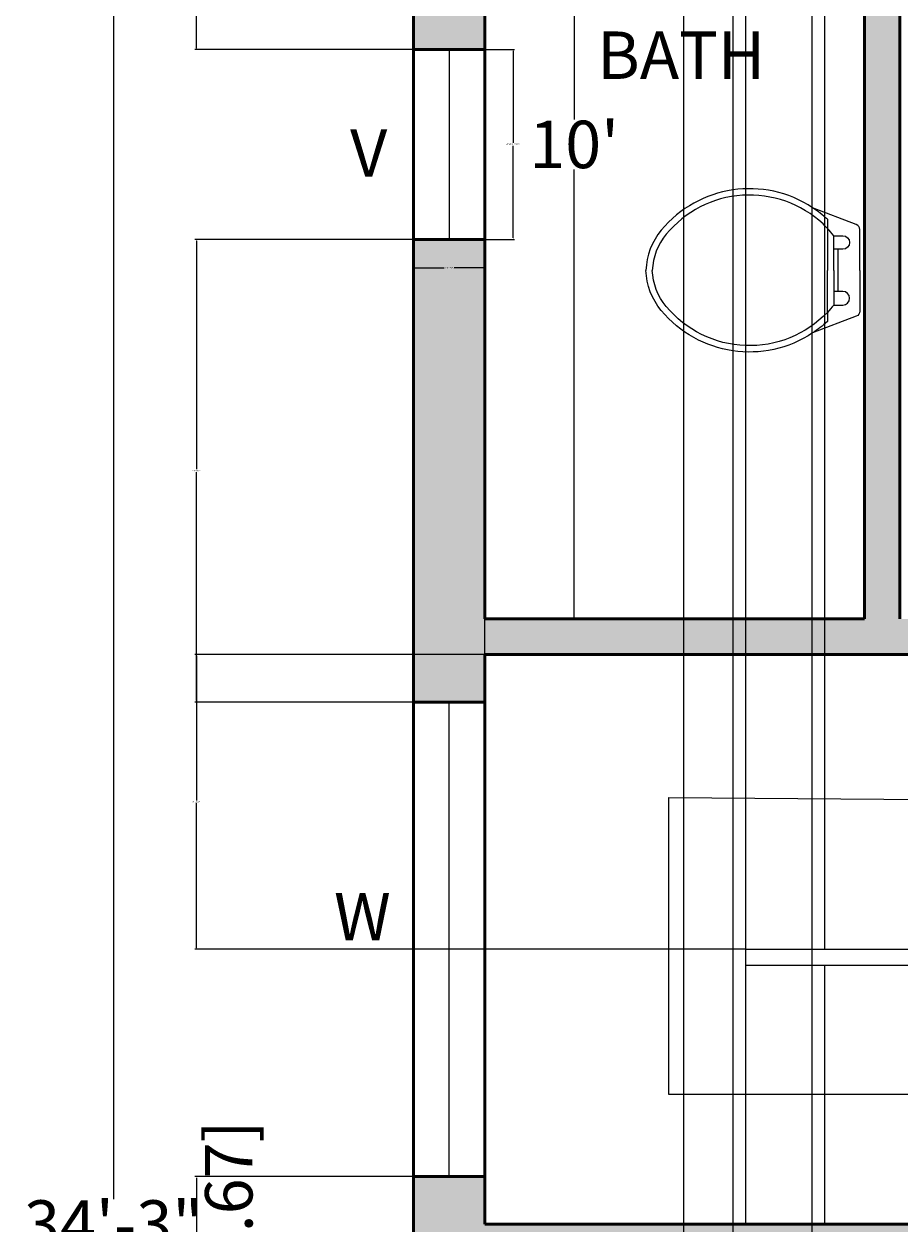
# Model space of a CAD drawing. Units: inches. Extents: x -22 to 470, y -437 to 97.
# Tile 5 of 9: x -22 to 88, y -192 to -41. Entities that reach past the tile are written whole.
import ezdxf

# ---------------------------------------------------------------- set-up
doc = ezdxf.new("R2010")
doc.units = ezdxf.units.IN
doc.header["$MEASUREMENT"] = 0
for name, color, linetype, lineweight in [('A-ANNO-DIMS', 2, 'Continuous', 18), ('A-ANNO-TEXT', 7, 'Continuous', 18), ('A-AREA-IDEN', 7, 'Continuous', 25), ('A-FLOR-FIXT', 9, 'Continuous', 20), ('A-FLOR-STRS', 7, 'Continuous', 25), ('A-GLAZ', 4, 'Continuous', 18), ('A-WALL', 7, 'Continuous', 50), ('A-WALL-PATT', 8, 'Continuous', 13)]:
    doc.layers.add(name, color=color, linetype=linetype, lineweight=lineweight)
doc.styles.get("Standard").update_dxf_attribs({"font": 'arial.ttf'})
doc.dimstyles.get("Standard").update_dxf_attribs({"dimtxt": 0.18, "dimasz": 0.18, "dimexe": 0.18, "dimexo": 0.0625, "dimgap": 0.09, "dimtad": 0, "dimtih": 1, "dimtoh": 1, "dimdec": 0, "dimzin": 0, "dimdsep": 46, "dimlunit": 3, "dimtxsty": 'Standard', "dimcen": 0.09, "dimadec": 0, "dimazin": 0, "dimtfac": 1, "dimtdec": 0, "dimtofl": 0, "dimtmove": 0, "dimatfit": 3, "dimfxl": 1, "dimtolj": 1, "dimtzin": 0, "dimarcsym": 0})

# ---------------------------------------------------------------- blocks, each defined once
blk = doc.blocks.new('*D3')
at = {"layer": 'A-ANNO-DIMS', "color": 0, "lineweight": -2, "transparency": 16777216}
for p, q in [((26.86, 13.24), (-11.18, 13.24)), ((-11, 13.06), (-11, -189.1)), ((-11, -397.58), (-11, -195.41)), ((26.86, -397.76), (-11.18, -397.76))]:
    blk.add_line(p, q, dxfattribs=at)
at = {"layer": 'A-ANNO-DIMS', "color": 0, "transparency": 16777216}
for points in [[(-11.03, 13.06), (-10.97, 13.06), (-11, 13.24)], [(-11.03, -397.58), (-10.97, -397.58), (-11, -397.76)]]:
    blk.add_solid(points, dxfattribs=at)
at = {"layer": 'Defpoints', "color": 0, "transparency": 16777216}
for p in [(26.92, 13.24), (-11, -397.76), (26.92, -397.76)]:
    blk.add_point(p, dxfattribs=at)
at = {"layer": 'A-ANNO-DIMS', "color": 0, "transparency": 16777216, "insert": (-11, -192.26), "char_height": 6, "attachment_point": 5}
blk.add_mtext('\\A1;34\'-3"', dxfattribs=at)
blk = doc.blocks.new('*D5')
at = {"layer": 'A-ANNO-DIMS', "color": 0, "lineweight": -2, "transparency": 16777216}
for p, q in [((47.18, 4.24), (47.06, 4.24)), ((47.24, 4.06), (47.24, -52.6)), ((47.24, -115.58), (47.24, -58.91)), ((47.18, -115.76), (47.06, -115.76))]:
    blk.add_line(p, q, dxfattribs=at)
at = {"layer": 'A-ANNO-DIMS', "color": 0, "transparency": 16777216}
for points in [[(47.21, 4.06), (47.27, 4.06), (47.24, 4.24)], [(47.21, -115.58), (47.27, -115.58), (47.24, -115.76)]]:
    blk.add_solid(points, dxfattribs=at)
at = {"layer": 'Defpoints', "color": 0, "transparency": 16777216}
for p in [(47.24, 4.24), (47.24, 4.24), (47.24, -115.76)]:
    blk.add_point(p, dxfattribs=at)
at = {"layer": 'A-ANNO-DIMS', "color": 0, "transparency": 16777216, "insert": (47.24, -55.76), "char_height": 6, "attachment_point": 5}
blk.add_mtext("\\A1;10'", dxfattribs=at)
blk = doc.blocks.new('WC-PLAN')
for p, q in [((22.94, 16.78), (22.94, 15.64)), ((22.94, 15.64), (22.94, 10.33)), ((22.94, 5.01), (22.94, 10.33)), ((22.94, 5.01), (22.94, 3.87))]:
    blk.add_line(p, q)
for points in [[(21.08, 18.24, 0.383919), (1.95, 15.41, 0.163732), (0, 10.33, 0.359733)], [(22.39, 16.19, 0.431639), (2.57, 14.89, 0.162618), (0.81, 10.33, 0.470877)], [(22.94, 16.78, 0.040937), (21.08, 18.24, 0.163732)], [(27.03, 10.33), (27.03, 15.49, 0.31031), (26.6, 16.12), (21.08, 18.24, 0.209071)], [(22.94, 15.64, 0.014165), (22.39, 16.19, 0.162618)], [(23.75, 14.71, 0.022712), (22.94, 15.64, 0.162618)], [(23.75, 10.33), (23.75, 14.71, 0.022712)], [(23.75, 14.71), (24.89, 14.71, -1), (24.89, 12.99), (24.3, 12.99)], [(21.08, 2.41, -0.383919), (1.95, 5.25, -0.163732), (0, 10.33, -0.359733)], [(22.94, 5.01, -0.448546), (2.57, 5.76, -0.162618), (0.81, 10.33, -0.470877)], [(27.03, 10.33), (27.03, 5.16, -0.31031), (26.6, 4.53), (21.08, 2.41, -0.209071)], [(23.75, 10.33), (23.75, 5.94, -0.476108)], [(23.75, 5.94), (24.89, 5.94, 1), (24.89, 7.67), (24.3, 7.67)], [(23.75, 5.94, -0.022712), (22.94, 5.01, -0.162618)], [(22.94, 3.87, -0.040937), (21.08, 2.41, -0.163732)]]:
    blk.add_lwpolyline(points, format="xyb")
for points in [[(24.3, 12.99), (23.75, 12.99)], [(24.3, 7.67), (24.3, 12.99)], [(24.3, 7.67), (23.75, 7.67)]]:
    blk.add_lwpolyline(points)
blk = doc.blocks.new('WINDOW-60-SASH')
for p, q in [((0, 9), (60, 9)), ((0, 4.5), (60, 4.5)), ((60, 0), (0, 0))]:
    blk.add_line(p, q)
blk = doc.blocks.new('VENT-24-SASH')
for p, q in [((0, 24), (0, 0)), ((4.5, 24), (4.5, 0)), ((9, 0), (9, 24))]:
    blk.add_line(p, q)
blk = doc.blocks.new('*D39')
at = {"layer": 'A-ANNO-DIMS', "color": 0, "lineweight": -2, "transparency": 16777216}
for p, q in [((35.98, -43.76), (39.7, -43.76)), ((39.52, -43.94), (39.52, -55.57)), ((39.52, -67.58), (39.52, -55.94)), ((35.98, -67.76), (39.7, -67.76))]:
    blk.add_line(p, q, dxfattribs=at)
at = {"layer": 'A-ANNO-DIMS', "color": 0, "transparency": 16777216}
for points in [[(39.49, -43.94), (39.55, -43.94), (39.52, -43.76)], [(39.49, -67.58), (39.55, -67.58), (39.52, -67.76)]]:
    blk.add_solid(points, dxfattribs=at)
at = {"layer": 'Defpoints', "color": 0, "transparency": 16777216}
for p in [(35.92, -43.76), (39.52, -43.76), (35.92, -67.76)]:
    blk.add_point(p, dxfattribs=at)
at = {"layer": 'A-ANNO-DIMS', "color": 0, "transparency": 16777216, "insert": (39.52, -55.76), "char_height": 0.18, "attachment_point": 5}
blk.add_mtext('\\A1;VENT 2\'-0" TYP.', dxfattribs=at)
blk = doc.blocks.new('*D40')
at = {"layer": 'A-ANNO-DIMS', "color": 0, "lineweight": -2, "transparency": 16777216}
for p, q in [((26.92, -67.82), (26.92, -71.54)), ((35.92, -67.82), (35.92, -71.54)), ((27.1, -71.36), (30.78, -71.36)), ((35.74, -71.36), (32.06, -71.36))]:
    blk.add_line(p, q, dxfattribs=at)
at = {"layer": 'A-ANNO-DIMS', "color": 0, "transparency": 16777216}
for points in [[(27.1, -71.33), (27.1, -71.39), (26.92, -71.36)], [(35.74, -71.33), (35.74, -71.39), (35.92, -71.36)]]:
    blk.add_solid(points, dxfattribs=at)
at = {"layer": 'Defpoints', "color": 0, "transparency": 16777216}
for p in [(26.92, -67.76), (35.92, -67.76), (35.92, -71.36)]:
    blk.add_point(p, dxfattribs=at)
at = {"layer": 'A-ANNO-DIMS', "color": 0, "transparency": 16777216, "insert": (31.42, -71.36), "char_height": 0.18, "attachment_point": 5}
blk.add_mtext('\\A1;0\'-9" TYP.', dxfattribs=at)
blk = doc.blocks.new('*D63')
at = {"layer": 'A-ANNO-DIMS', "color": 0, "lineweight": -2, "transparency": 16777216}
for p, q in [((68.92, -120.19), (68.92, 40.87)), ((69.1, 40.69), (73.52, 40.69)), ((78.74, 40.69), (74.32, 40.69)), ((78.92, -120.19), (78.92, 40.87))]:
    blk.add_line(p, q, dxfattribs=at)
at = {"layer": 'A-ANNO-DIMS', "color": 0, "transparency": 16777216}
for points in [[(69.1, 40.72), (69.1, 40.66), (68.92, 40.69)], [(78.74, 40.72), (78.74, 40.66), (78.92, 40.69)]]:
    blk.add_solid(points, dxfattribs=at)
at = {"layer": 'Defpoints', "color": 0, "transparency": 16777216}
for p in [(78.92, 40.69), (68.92, -120.26), (78.92, -120.26)]:
    blk.add_point(p, dxfattribs=at)
at = {"layer": 'A-ANNO-DIMS', "color": 0, "transparency": 16777216, "insert": (73.92, 40.69), "char_height": 0.18, "attachment_point": 5}
blk.add_mtext('\\A1;0\'-10"', dxfattribs=at)
blk = doc.blocks.new('*D67')
at = {"layer": 'A-ANNO-DIMS', "color": 0, "lineweight": -2, "transparency": 16777216}
for p, q in [((26.86, 13.24), (-0.71, 13.24)), ((-0.53, 13.06), (-0.53, -15.07)), ((-0.53, -43.58), (-0.53, -15.44)), ((26.86, -43.76), (-0.71, -43.76))]:
    blk.add_line(p, q, dxfattribs=at)
at = {"layer": 'A-ANNO-DIMS', "color": 0, "transparency": 16777216}
for points in [[(-0.56, 13.06), (-0.5, 13.06), (-0.53, 13.24)], [(-0.56, -43.58), (-0.5, -43.58), (-0.53, -43.76)]]:
    blk.add_solid(points, dxfattribs=at)
at = {"layer": 'Defpoints', "color": 0, "transparency": 16777216}
for p in [(26.92, 13.24), (-0.53, -43.76), (26.92, -43.76)]:
    blk.add_point(p, dxfattribs=at)
at = {"layer": 'A-ANNO-DIMS', "color": 0, "transparency": 16777216, "insert": (-0.53, -15.26), "char_height": 0.18, "attachment_point": 5}
blk.add_mtext('\\A1;4\'-9"', dxfattribs=at)
blk = doc.blocks.new('*D68')
at = {"layer": 'A-ANNO-DIMS', "color": 0, "lineweight": -2, "transparency": 16777216}
for p, q in [((26.86, -67.76), (-0.71, -67.76)), ((-0.53, -67.94), (-0.53, -96.82)), ((-0.53, -126.08), (-0.53, -97.19)), ((26.86, -126.26), (-0.71, -126.26))]:
    blk.add_line(p, q, dxfattribs=at)
at = {"layer": 'A-ANNO-DIMS', "color": 0, "transparency": 16777216}
for points in [[(-0.56, -67.94), (-0.5, -67.94), (-0.53, -67.76)], [(-0.56, -126.08), (-0.5, -126.08), (-0.53, -126.26)]]:
    blk.add_solid(points, dxfattribs=at)
at = {"layer": 'Defpoints', "color": 0, "transparency": 16777216}
for p in [(26.92, -67.76), (-0.53, -126.26), (26.92, -126.26)]:
    blk.add_point(p, dxfattribs=at)
at = {"layer": 'A-ANNO-DIMS', "color": 0, "transparency": 16777216, "insert": (-0.53, -97.01), "char_height": 0.18, "attachment_point": 5}
blk.add_mtext('\\A1;4\'-10 1/2"', dxfattribs=at)
blk = doc.blocks.new('*D69')
at = {"layer": 'A-ANNO-DIMS', "color": 0, "lineweight": -2, "transparency": 16777216}
for p, q in [((26.86, -186.26), (-0.71, -186.26)), ((-0.53, -186.44), (-0.53, -205.07)), ((-0.53, -224.07), (-0.53, -205.44)), ((26.86, -224.25), (-0.71, -224.25))]:
    blk.add_line(p, q, dxfattribs=at)
at = {"layer": 'A-ANNO-DIMS', "color": 0, "transparency": 16777216}
for points in [[(-0.56, -186.44), (-0.5, -186.44), (-0.53, -186.26)], [(-0.56, -224.07), (-0.5, -224.07), (-0.53, -224.25)]]:
    blk.add_solid(points, dxfattribs=at)
at = {"layer": 'Defpoints', "color": 0, "transparency": 16777216}
for p in [(26.92, -186.26), (-0.53, -224.25), (26.92, -224.25)]:
    blk.add_point(p, dxfattribs=at)
at = {"layer": 'A-ANNO-DIMS', "color": 0, "transparency": 16777216, "insert": (-0.53, -205.25), "char_height": 0.18, "attachment_point": 5}
blk.add_mtext('\\A1;3\'-2"', dxfattribs=at)
blk = doc.blocks.new('*D77')
at = {"layer": 'A-ANNO-DIMS', "color": 0, "lineweight": -2, "transparency": 16777216}
for p, q in [((68.86, -120.26), (-0.71, -120.26)), ((-0.53, -120.44), (-0.53, -138.7)), ((-0.53, -157.33), (-0.53, -139.06)), ((68.86, -157.51), (-0.71, -157.51))]:
    blk.add_line(p, q, dxfattribs=at)
at = {"layer": 'A-ANNO-DIMS', "color": 0, "transparency": 16777216}
for points in [[(-0.56, -120.44), (-0.5, -120.44), (-0.53, -120.26)], [(-0.56, -157.33), (-0.5, -157.33), (-0.53, -157.51)]]:
    blk.add_solid(points, dxfattribs=at)
at = {"layer": 'Defpoints', "color": 0, "transparency": 16777216}
for p in [(68.92, -120.26), (-0.53, -157.51), (68.92, -157.51)]:
    blk.add_point(p, dxfattribs=at)
at = {"layer": 'A-ANNO-DIMS', "color": 0, "transparency": 16777216, "insert": (-0.53, -138.88), "char_height": 0.18, "attachment_point": 5}
blk.add_mtext('\\A1;3\'-1 1/2"', dxfattribs=at)
blk = doc.blocks.new('*D78')
at = {"layer": 'A-ANNO-DIMS', "color": 0, "lineweight": -2, "transparency": 16777216}
for p, q in [((35.92, -192.19), (35.92, 40.87)), ((36.1, 40.69), (52.09, 40.69)), ((68.74, 40.69), (52.75, 40.69)), ((68.92, -192.19), (68.92, 40.87))]:
    blk.add_line(p, q, dxfattribs=at)
at = {"layer": 'A-ANNO-DIMS', "color": 0, "transparency": 16777216}
for points in [[(36.1, 40.72), (36.1, 40.66), (35.92, 40.69)], [(68.74, 40.72), (68.74, 40.66), (68.92, 40.69)]]:
    blk.add_solid(points, dxfattribs=at)
at = {"layer": 'Defpoints', "color": 0, "transparency": 16777216}
for p in [(68.92, 40.69), (35.92, -192.26), (68.92, -192.26)]:
    blk.add_point(p, dxfattribs=at)
at = {"layer": 'A-ANNO-DIMS', "color": 0, "transparency": 16777216, "insert": (52.42, 40.69), "char_height": 0.18, "attachment_point": 5}
blk.add_mtext('\\A1;2\'-9"', dxfattribs=at)
blk = doc.blocks.new('*D79')
at = {"layer": 'A-ANNO-DIMS', "color": 0, "lineweight": -2, "transparency": 16777216}
for p, q in [((61.08, -228.48), (61.08, 40.87)), ((61.26, 40.69), (93.66, 40.69)), ((126.72, 40.69), (94.32, 40.69)), ((126.9, -228.48), (126.9, 40.87))]:
    blk.add_line(p, q, dxfattribs=at)
at = {"layer": 'A-ANNO-DIMS', "color": 0, "transparency": 16777216}
for points in [[(61.26, 40.72), (61.26, 40.66), (61.08, 40.69)], [(126.72, 40.72), (126.72, 40.66), (126.9, 40.69)]]:
    blk.add_solid(points, dxfattribs=at)
at = {"layer": 'Defpoints', "color": 0, "transparency": 16777216}
for p in [(126.9, 40.69), (61.08, -228.55), (126.9, -228.55)]:
    blk.add_point(p, dxfattribs=at)
at = {"layer": 'A-ANNO-DIMS', "color": 0, "transparency": 16777216, "insert": (93.99, 40.69), "char_height": 0.18, "attachment_point": 5}
blk.add_mtext('\\A1;5\'-6"', dxfattribs=at)
blk = doc.blocks.new('*D83')
at = {"layer": 'A-ANNO-DIMS', "color": 0, "lineweight": -2, "transparency": 16777216}
for p, q in [((67.35, -370.26), (67.35, 40.87)), ((67.53, 40.69), (71.94, 40.69)), ((77.15, 40.69), (72.74, 40.69)), ((77.33, -369.14), (77.33, 40.87))]:
    blk.add_line(p, q, dxfattribs=at)
at = {"layer": 'A-ANNO-DIMS', "color": 0, "transparency": 16777216}
for points in [[(67.53, 40.72), (67.53, 40.66), (67.35, 40.69)], [(77.15, 40.72), (77.15, 40.66), (77.33, 40.69)]]:
    blk.add_solid(points, dxfattribs=at)
at = {"layer": 'Defpoints', "color": 0, "transparency": 16777216}
for p in [(77.33, 40.69), (77.33, -369.2), (67.35, -370.32)]:
    blk.add_point(p, dxfattribs=at)
at = {"layer": 'A-ANNO-DIMS', "color": 0, "transparency": 16777216, "insert": (72.34, 40.69), "char_height": 0.18, "attachment_point": 5}
blk.add_mtext('\\A1;0\'-10"', dxfattribs=at)

msp = doc.modelspace()

# ---------------------------------------------------------------- hatches: boundary and pattern name
at = {"layer": 'A-WALL-PATT'}
h = msp.add_hatch(color=256, dxfattribs=at)
h.dxf.hatch_style = 1
h.paths.add_polyline_path([(130.42, 13.24), (26.92, 13.24), (26.92, -43.76), (35.92, -43.76), (35.92, 4.24), (83.92, 4.24), (83.92, 1.24), (88.42, 1.24), (88.42, 4.24), (130.42, 4.24)])
h.paths.add_polyline_path([(266.92, 13.24), (190.42, 13.24), (190.42, 4.24), (232.42, 4.24), (232.42, -115.76), (229.42, -115.76), (229.42, -120.26), (239.92, -120.26), (239.92, -115.76), (236.92, -115.76), (236.92, 4.24), (266.92, 4.24)])
h.paths.add_polyline_path([(442.42, 13.24), (326.92, 13.24), (326.92, 4.24), (356.92, 4.24), (356.92, 1.24), (361.42, 1.24), (361.42, 4.24), (433.42, 4.24), (433.42, -49.38), (442.42, -49.38)])
h.paths.add_polyline_path([(442.42, -73.38), (433.42, -73.38), (433.42, -115.76), (361.42, -115.76), (361.42, -22.76), (356.92, -22.76), (356.92, -115.76), (263.92, -115.76), (263.92, -120.26), (332.92, -120.26), (332.92, -123.26), (337.42, -123.26), (337.42, -120.26), (433.42, -120.26), (433.42, -148.49), (442.42, -148.49)])
h.paths.add_polyline_path([(205.42, -115.76), (88.42, -115.76), (88.42, -22.76), (83.92, -22.76), (83.92, -115.76), (35.92, -115.76), (35.92, -67.76), (26.92, -67.76), (26.92, -126.26), (35.92, -126.26), (35.92, -120.26), (205.42, -120.26)])
h.paths.add_polyline_path([(35.92, -196.76), (168.92, -196.76), (168.92, -192.26), (35.92, -192.26), (35.92, -186.26), (26.92, -186.26), (26.92, -224.25), (35.92, -224.25)])
h.paths.add_polyline_path([(35.92, -284.25), (26.92, -284.25), (26.92, -397.76), (53.92, -397.76), (53.92, -388.76), (35.92, -388.76)])
h.paths.add_polyline_path([(142.42, -388.76), (136.42, -388.76), (136.42, -316.76), (181.42, -316.76), (181.42, -312.26), (136.42, -312.26), (136.42, -303.75), (131.92, -303.75), (131.92, -388.76), (113.92, -388.76), (113.92, -397.76), (142.42, -397.76)])
h.paths.add_polyline_path([(218.92, -388.76), (212.92, -388.76), (212.92, -312.26), (205.42, -312.26), (205.42, -316.76), (208.42, -316.76), (208.42, -388.76), (202.42, -388.76), (202.42, -397.76), (218.92, -397.76)])
h.paths.add_polyline_path([(306.75, -388.76), (289.42, -388.76), (289.42, -316.76), (284.92, -316.76), (284.92, -388.76), (278.92, -388.76), (278.92, -397.76), (306.75, -397.76)])
h.paths.add_polyline_path([(391.42, -388.76), (366.75, -388.76), (366.75, -397.76), (391.42, -397.76)], flags=17)
h.paths.add_polyline_path([(442.42, -172.49), (433.42, -172.49), (433.42, -192.26), (337.42, -192.26), (337.42, -147.26), (332.92, -147.26), (332.92, -196.76), (433.42, -196.76), (433.42, -388.76), (427.42, -388.76), (427.42, -397.76), (442.42, -397.76)])

# ---------------------------------------------------------------- linework, layer by layer
at = {"layer": 'A-FLOR-STRS'}
for p, q in [((68.92, -192.26), (68.92, -120.26)), ((78.92, -157.51), (78.92, -120.26)), ((59.19, -175.88), (59.19, -138.35)), ((59.19, -138.35), (128.92, -138.88)), ((68.92, -157.51), (168.92, -157.51)), ((68.92, -159.51), (168.92, -159.51)), ((78.92, -192.26), (78.92, -159.51)), ((138.92, -175.88), (59.19, -175.88))]:
    msp.add_line(p, q, dxfattribs=at)
at = {"layer": 'A-WALL'}
for p, q in [((26.92, 13.24), (26.92, -397.76)), ((35.92, 4.24), (35.92, -115.76)), ((88.42, 4.24), (88.42, -115.76)), ((83.92, -22.76), (83.92, -115.76)), ((35.92, -43.76), (26.92, -43.76)), ((26.92, -67.76), (35.92, -67.76)), ((35.92, -115.76), (83.92, -115.76)), ((35.92, -120.26), (332.92, -120.26)), ((35.92, -120.26), (35.92, -192.26)), ((35.92, -126.26), (26.92, -126.26)), ((26.92, -186.26), (35.92, -186.26)), ((168.92, -192.26), (35.92, -192.26))]:
    msp.add_line(p, q, dxfattribs=at)

# ---------------------------------------------------------------- block references
at = {"layer": 'A-FLOR-FIXT'}
msp.add_blockref('WC-PLAN', (56.3, -82.01), dxfattribs=at)
at = {"layer": 'A-GLAZ'}
msp.add_blockref('VENT-24-SASH', (26.92, -67.76), dxfattribs=at)
at = {"layer": 'A-GLAZ', "rotation": 90.00000000000003}
msp.add_blockref('WINDOW-60-SASH', (35.92, -186.26), dxfattribs=at)

# ---------------------------------------------------------------- texts
at = {"layer": 'A-ANNO-DIMS', "insert": (0.57, -205.16), "char_height": 6, "attachment_point": 1, "rotation": 90}
msp.add_mtext('[10.67]', dxfattribs=at)
at = {"layer": 'A-ANNO-TEXT', "insert": (18.9, -53.84), "char_height": 6, "attachment_point": 1}
msp.add_mtext_dynamic_manual_height_columns('V', width=1.9846, gutter_width=1, heights=[0], dxfattribs=at)
at = {"layer": 'A-ANNO-TEXT', "insert": (16.87, -150.39), "char_height": 6, "attachment_point": 1}
msp.add_mtext('W', dxfattribs=at)
at = {"layer": 'A-AREA-IDEN', "insert": (50.15, -41.48), "char_height": 6, "attachment_point": 1}
msp.add_mtext('BATH', dxfattribs=at)

# ---------------------------------------------------------------- dimensions: what is measured, and where the dimension line sits
at = {"layer": 'A-ANNO-DIMS'}
for base, p1, p2, picture, middle in [((68.92, 40.69), (35.92, -192.26), (68.92, -192.26), '*D78', (52.42, 40.69)), ((126.9, 40.69), (61.08, -228.55), (126.9, -228.55), '*D79', (93.99, 40.69)), ((77.33, 40.69), (67.35, -370.32), (77.33, -369.2), '*D83', (72.34, 40.69)), ((78.92, 40.69), (68.92, -120.26), (78.92, -120.26), '*D63', (73.92, 40.69))]:
    dim = msp.add_linear_dim(base=base, p1=p1, p2=p2, dimstyle='Standard', override={"dimdec": 1, "dimlfac": 1, "dimrnd": 0, "dimzin": 1, "dimdsep": 46, "dimlunit": 4, "dimfrac": 2}, dxfattribs=at)
    dim.commit()
    dim.dimension.update_dxf_attribs({"geometry": picture, "text_midpoint": middle})
for base, p1, p2, override, picture, middle in [((-11, -397.76), (26.92, 13.24), (26.92, -397.76), {"dimtxt": 6, "dimclrd": 0, "dimclre": 0, "dimclrt": 0}, '*D3', (-11, -192.26)), ((-0.53, -43.76), (26.92, 13.24), (26.92, -43.76), {"dimdec": 1, "dimlfac": 1, "dimrnd": 0, "dimzin": 1, "dimdsep": 46, "dimlunit": 4, "dimfrac": 2}, '*D67', (-0.53, -15.26)), ((47.24, 4.24), (47.24, -115.76), (47.24, 4.24), {"dimtxt": 6, "dimclrd": 0, "dimclre": 0, "dimclrt": 0}, '*D5', (47.24, -55.76)), ((-0.53, -126.26), (26.92, -67.76), (26.92, -126.26), {"dimdec": 1, "dimlfac": 1, "dimrnd": 0, "dimzin": 1, "dimdsep": 46, "dimlunit": 4, "dimfrac": 2}, '*D68', (-0.53, -97.01)), ((-0.528386, -157.506367), (68.921614, -120.256367), (68.921614, -157.506367), {"dimdec": 1, "dimlfac": 1, "dimrnd": 0, "dimzin": 1, "dimdsep": 46, "dimlunit": 4, "dimfrac": 2}, '*D77', (-0.528386, -138.881367)), ((-0.53, -224.25), (26.92, -186.26), (26.92, -224.25), {"dimdec": 1, "dimlfac": 1, "dimrnd": 0, "dimzin": 1, "dimdsep": 46, "dimlunit": 4, "dimfrac": 2}, '*D69', (-0.53, -205.25))]:
    dim = msp.add_linear_dim(base=base, p1=p1, p2=p2, angle=90, dimstyle='Standard', override=override, dxfattribs=at)
    dim.commit()
    dim.dimension.update_dxf_attribs({"geometry": picture, "text_midpoint": middle})
dim = msp.add_linear_dim(base=(39.52, -43.76), p1=(35.92, -67.76), p2=(35.92, -43.76), angle=90, text='VENT <> TYP.', dimstyle='Standard', override={"dimdec": 1, "dimlfac": 1, "dimrnd": 0, "dimzin": 1, "dimdsep": 46, "dimlunit": 4, "dimfrac": 2}, dxfattribs=at)
dim.commit()
dim.dimension.update_dxf_attribs({"geometry": '*D39', "text_midpoint": (39.52, -55.76)})
dim = msp.add_linear_dim(base=(35.92, -71.36), p1=(26.92, -67.76), p2=(35.92, -67.76), text='<> TYP.', dimstyle='Standard', override={"dimdec": 1, "dimlfac": 1, "dimrnd": 0, "dimzin": 1, "dimdsep": 46, "dimlunit": 4, "dimfrac": 2}, dxfattribs=at)
dim.commit()
dim.dimension.update_dxf_attribs({"geometry": '*D40', "text_midpoint": (31.42, -71.36)})

doc.saveas('drawing.dxf')
